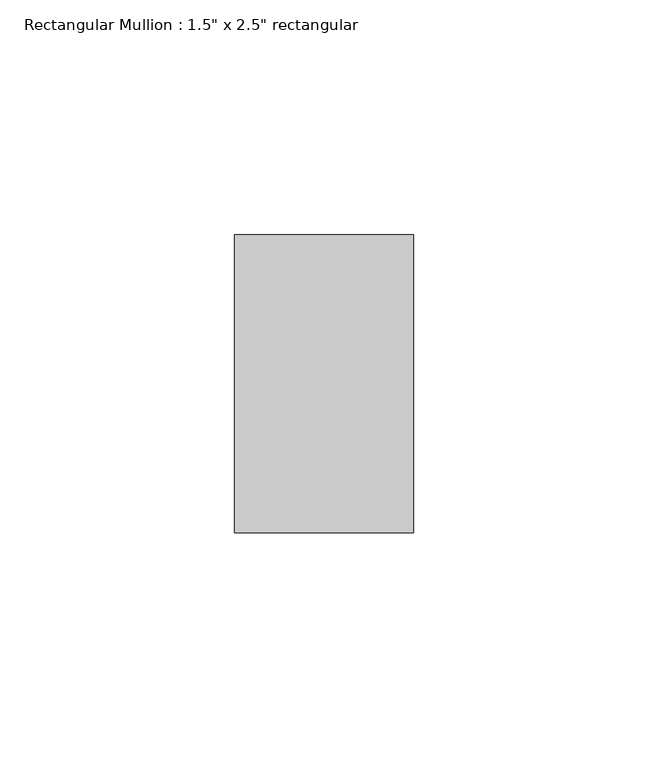
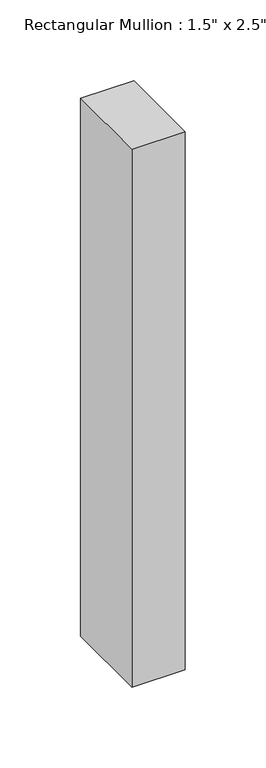
"""IFC4 building model written with IfcOpenShell, lengths in millimetres: member geometry."""

from ifc_helpers import new_model, si_unit, frame, origin, place, context, project, spatial, polyline, outline, extrude, source, transform, mapped, element, save


def member_54524429(model_context):
    return source(origin(), model_context, "Body", "SweptSolid", [
        extrude(outline(polyline([(19.05, 31.75), (19.05, -31.75), (-19.05, -31.75), (-19.05, 31.75), (19.05, 31.75)])), frame((0.0, 0.0, -406.4), z_axis=(0.0, 0.0, 1.0), x_axis=(1.0, 0.0, 0.0)), (0.0, 0.0, 1.0), 406.4),
    ])


if __name__ == "__main__":
    model = new_model("IFC4")
    model_context = context("Model", 3, world=origin())
    ifc_project = project(units=[si_unit("LENGTHUNIT", "METRE", prefix="MILLI")], contexts=[model_context])
    site = spatial("IfcSite", under=ifc_project)
    building = spatial("IfcBuilding", under=site)
    placement = place(None, origin())
    member_shape = member_54524429(model_context)
    element("IfcMember", 1, ObjectType="Rectangular Mullion : 1.5\" x 2.5\" rectangular", at=placement, inside=building, context=model_context, shape_type="MappedRepresentation", body=[
        mapped(member_shape, transform((0.0, 0.0, 0.0), x_axis=(1.0, 0.0, 0.0), y_axis=(0.0, 1.0, 0.0), z_axis=(0.0, 0.0, 1.0))),
    ])
    save(model, "model.ifc")

# Revit data of these elements
# Type "Rectangular Mullion : 1.5\" x 2.5\" rectangular"
#   built-in parameter 1007304 = 0.208333 (stored number, unit not read)
#   built-in parameter 1007301 = 0.0625 (stored number, unit not read)
#   built-in parameter 1007300 = 0.0625 (stored number, unit not read)
# Element 1 (IfcMember, "Rectangular Mullion : 1.5\" x 2.5\" rectangular")
#   Materials on its faces: "Damp-proofing"
# Materials
#   "Damp-proofing": class "Generic", colour RGB 127 127 127, transparency 0, Description = "Damp-proofing", Cost = 0
